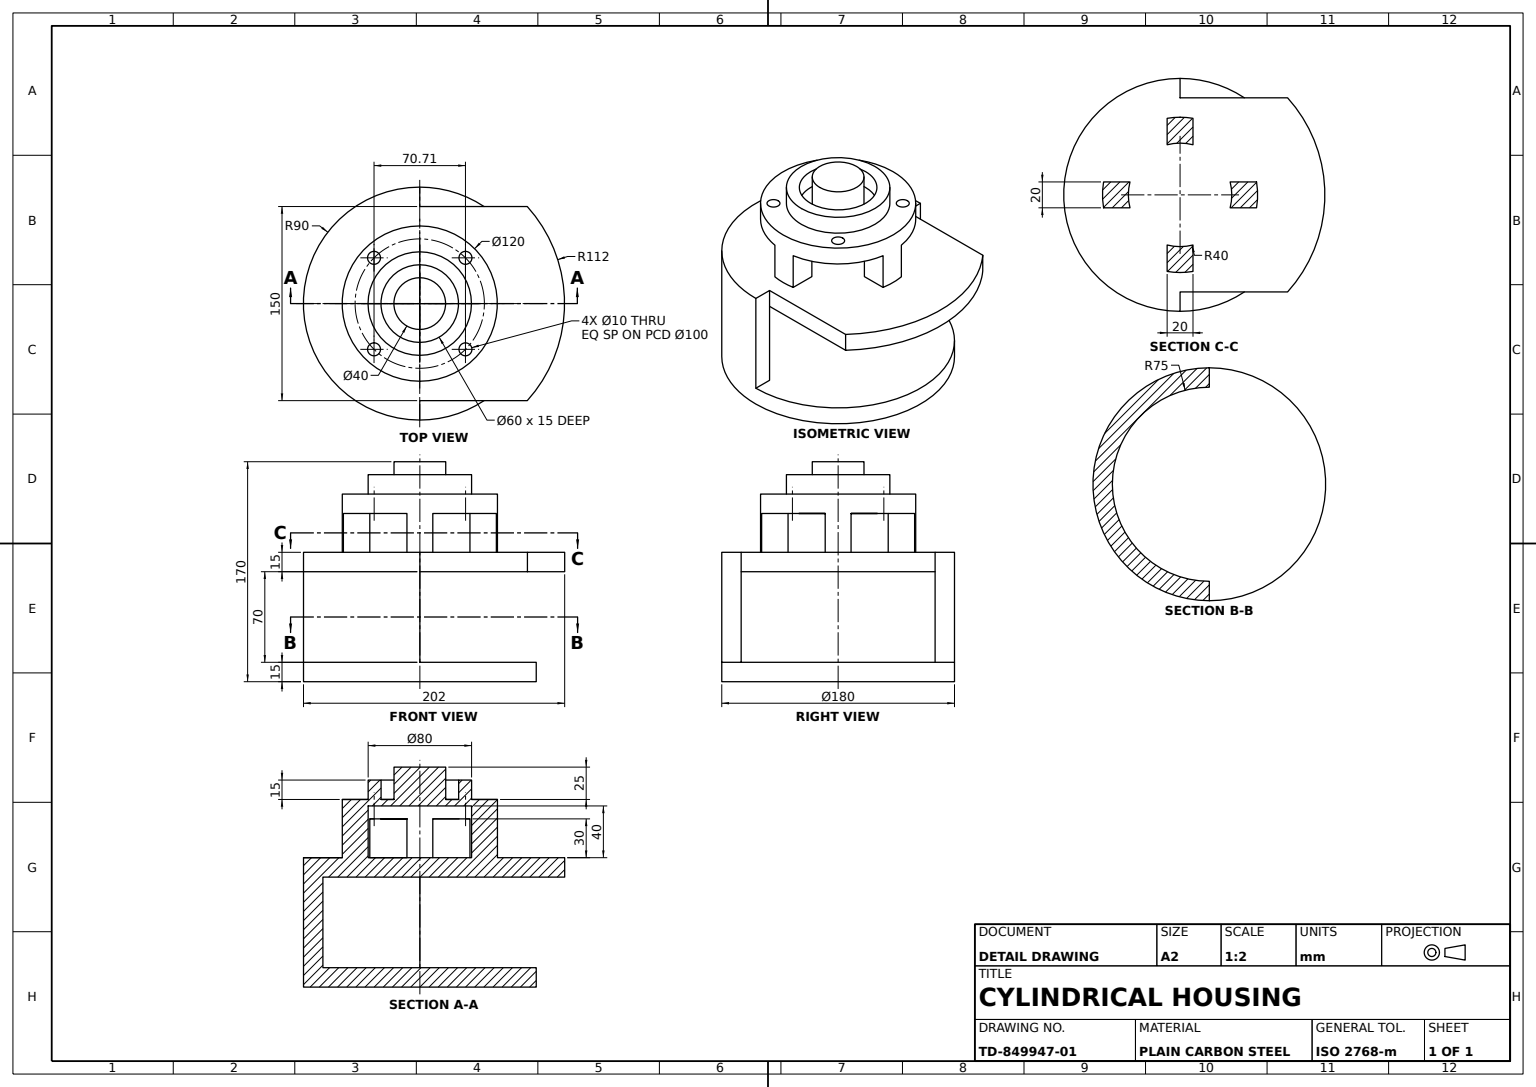
from build123d import *

# Parameters (mm, degrees)
BASE_DISC_SKETCH_R           = 90
BASE_DISC_180_DEPTH          = 15
CLAMP_FRAME_WALL_DEPTH       = 70
TOP_JAW_PLATE_DEPTH          = 15
TABLE_RISER_SKETCH_R         = 60
TABLE_RISER_SKETCH_R_2       = 40
TABLE_RISER_DEPTH            = 40
RISER_START                  = -30
RISER_SLOTS_CUT_DEPTH        = 30
TABLE_PLATE_SKETCH_R         = 60
TABLE_PLATE_120_DEPTH        = 5
TABLE_BOLT_HOLES_SKETCH_R    = 5
TABLE_BOLT_HOLES_4X_10_DEPTH = 20
TABLE_RING_SKETCH_R          = 40
TABLE_RING_SKETCH_R_2        = 30
TABLE_RING_80_DEPTH          = 15
CENTRE_SPIGOT_SKETCH_R       = 20
CENTRE_SPIGOT_40_DEPTH       = 25


with BuildPart() as part:
    # Base Disc Sketch → Base Disc Ø180 (new body)
    with BuildSketch(Plane(origin=(0, 0, 0), x_dir=(1, 0, 0), z_dir=(0, 1, 0))):
        with Locations(Location((0, 0, 0), (0, 0, 270))):
            Circle(BASE_DISC_SKETCH_R)
    extrude(amount=BASE_DISC_180_DEPTH)

    # Clamp Frame Wall Sketch → Clamp Frame Wall (add)
    with BuildSketch(Plane(origin=(0, 15, 0), x_dir=(1, 0, 0), z_dir=(0, 1, 0))):
        with BuildLine():
            Line((0, -90), (0, -75))
            ThreePointArc((0, -75), (-75, 0), (0, 75))
            Line((0, 75), (0, 90))
            ThreePointArc((0, 90), (-90, 0), (0, -90))
        make_face()
    extrude(amount=CLAMP_FRAME_WALL_DEPTH)

    # Top Jaw Sketch → Top Jaw Plate (add)
    with BuildSketch(Plane(origin=(0, 85, 0), x_dir=(1, 0, 0), z_dir=(0, 1, 0))):
        with BuildLine():
            Line((0, 75), (0, 90))
            ThreePointArc((0, 90), (-90, 0), (0, -90))
            Line((0, -90), (0, -75))
            ThreePointArc((0, -75), (-75, 0), (0, 75))
        make_face()
        with BuildLine():
            Line((0, -75), (0, 75))
            ThreePointArc((0, 75), (-75, 0), (0, -75))
        make_face()
        with BuildLine():
            Line((83.180526567, 75), (0, 75))
            Line((0, 75), (0, -75))
            Line((0, -75), (49.749371855, -75))
            Line((49.749371855, -75), (83.180526567, -75))
            ThreePointArc((83.180526567, -75), (112, 0), (83.180526567, 75))
        make_face()
    extrude(amount=TOP_JAW_PLATE_DEPTH)

    # Table Riser Sketch → Table Riser (add)
    with BuildSketch(Plane(origin=(0, 100, 0), x_dir=(1, 0, 0), z_dir=(0, 1, 0))):
        with Locations(Location((0, 0, 0), (0, 0, 270))):
            Circle(TABLE_RISER_SKETCH_R)
        with Locations(Location((0, 0, 0), (0, 0, 270))):
            Circle(TABLE_RISER_SKETCH_R_2, mode=Mode.SUBTRACT)
    extrude(amount=TABLE_RISER_DEPTH)

    # Riser Slots Sketch → Riser Slots Cut (cut)
    with BuildSketch(Plane(origin=(0, 130, 0), x_dir=(1, 0, 0), z_dir=(0, 1, 0)).offset(RISER_START)):
        with BuildLine():
            Line((59.160797831, 10), (38.729833462, 10))
            ThreePointArc((38.729833462, 10), (28.284271247, 28.284271247), (10, 38.729833462))
            Line((10, 38.729833462), (10, 59.160797831))
            ThreePointArc((10, 59.160797831), (42.426406871, 42.426406871), (59.160797831, 10))
        make_face()
        with BuildLine():
            Line((-10, 59.160797831), (-10, 38.729833462))
            ThreePointArc((-10, 38.729833462), (-28.284271247, 28.284271247), (-38.729833462, 10))
            Line((-38.729833462, 10), (-59.160797831, 10))
            ThreePointArc((-59.160797831, 10), (-42.426406871, 42.426406871), (-10, 59.160797831))
        make_face()
        with BuildLine():
            Line((59.160797831, -10), (38.729833462, -10))
            ThreePointArc((38.729833462, -10), (28.284271247, -28.284271247), (10, -38.729833462))
            Line((10, -38.729833462), (10, -59.160797831))
            ThreePointArc((10, -59.160797831), (42.426406871, -42.426406871), (59.160797831, -10))
        make_face()
        with BuildLine():
            Line((-10, -59.160797831), (-10, -38.729833462))
            ThreePointArc((-10, -38.729833462), (-28.284271247, -28.284271247), (-38.729833462, -10))
            Line((-38.729833462, -10), (-59.160797831, -10))
            ThreePointArc((-59.160797831, -10), (-42.426406871, -42.426406871), (-10, -59.160797831))
        make_face()
    extrude(amount=RISER_SLOTS_CUT_DEPTH, mode=Mode.SUBTRACT)

    # Table Plate Sketch → Table Plate Ø120 (add)
    with BuildSketch(Plane(origin=(0, 140, 0), x_dir=(1, 0, 0), z_dir=(0, 1, 0))):
        with Locations(Location((0, 0, 0), (0, 0, 80.405931773))):
            Circle(TABLE_PLATE_SKETCH_R)
    extrude(amount=TABLE_PLATE_120_DEPTH)

    # Table Bolt Holes Sketch → Table Bolt Holes 4xØ10 (cut)
    with BuildSketch(Plane(origin=(0, 145, 0), x_dir=(1, 0, 0), z_dir=(0, 1, 0))):
        with BuildLine():
            ThreePointArc((38.890872965, 38.890872965), (31.819805153, 38.890872965), (31.819805153, 31.819805153))
            Line((31.819805153, 31.819805153), (38.890872965, 38.890872965))
        make_face()
        with BuildLine():
            Line((38.890872965, 38.890872965), (31.819805153, 31.819805153))
            ThreePointArc((31.819805153, 31.819805153), (37.268756221, 30.735941397), (40.355339059, 35.355339059))
            ThreePointArc((40.355339059, 35.355339059), (39.974736722, 37.268756221), (38.890872965, 38.890872965))
        make_face()
        with Locations(Location((-35.355339059, 35.355339059, 0), (0, 0, 270))):
            Circle(TABLE_BOLT_HOLES_SKETCH_R)
        with Locations(Location((-35.355339059, -35.355339059, 0), (0, 0, 270))):
            Circle(TABLE_BOLT_HOLES_SKETCH_R)
        with Locations(Location((35.355339059, -35.355339059, 0), (0, 0, 270))):
            Circle(TABLE_BOLT_HOLES_SKETCH_R)
    extrude(amount=-TABLE_BOLT_HOLES_4X_10_DEPTH, mode=Mode.SUBTRACT)

    # Table Ring Sketch → Table Ring Ø80 (add)
    with BuildSketch(Plane(origin=(0, 145, 0), x_dir=(1, 0, 0), z_dir=(0, 1, 0))):
        with Locations(Location((0, 0, 0), (0, 0, 75.522487814))):
            Circle(TABLE_RING_SKETCH_R)
        with Locations(Location((0, 0, 0), (0, 0, 270))):
            Circle(TABLE_RING_SKETCH_R_2, mode=Mode.SUBTRACT)
    extrude(amount=TABLE_RING_80_DEPTH)

    # Centre Spigot Sketch → Centre Spigot Ø40 (add)
    with BuildSketch(Plane(origin=(0, 145, 0), x_dir=(1, 0, 0), z_dir=(0, 1, 0))):
        with Locations(Location((0, 0, 0), (0, 0, 270))):
            Circle(CENTRE_SPIGOT_SKETCH_R)
    extrude(amount=CENTRE_SPIGOT_40_DEPTH)


solid = part.part
